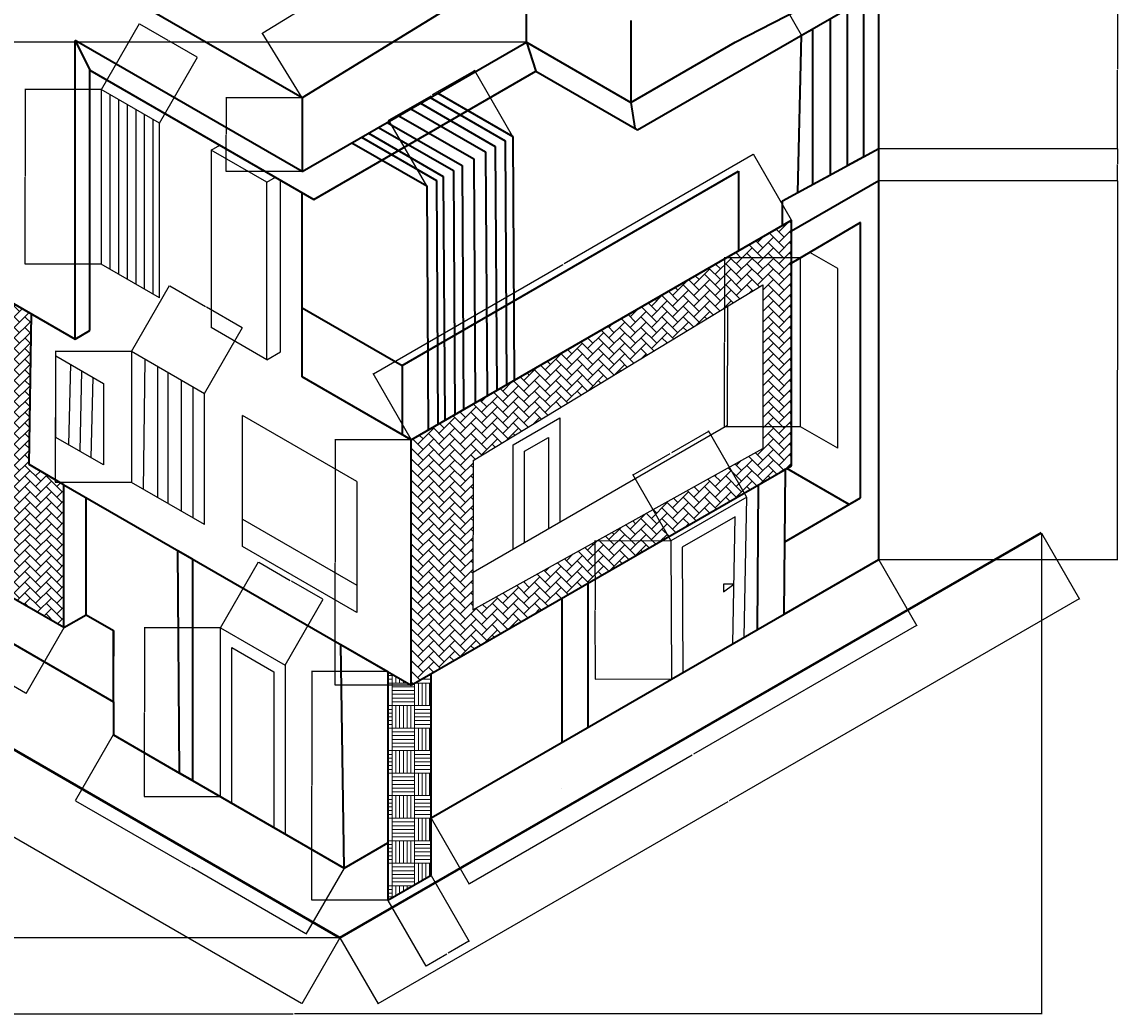
# Model space of a CAD drawing. Units: inches. Extents: x 61 to 939, y -128 to 676.
# Tile 2 of 3: x 355 to 939, y -128 to 400. Entities that reach past the tile are written whole.
import ezdxf

# ---------------------------------------------------------------- set-up
doc = ezdxf.new("R2010")
doc.units = ezdxf.units.IN
doc.header["$MEASUREMENT"] = 0
for name, color, linetype, lineweight in [('A-ANNO-DIMS', 2, 'Continuous', 18), ('A-DOOR', 3, 'Continuous', 25), ('A-ELEV', 7, 'Continuous', 35), ('A-GLAZ', 4, 'Continuous', 25), ('A-WALL-PATT', 8, 'Continuous', 18), ('C-TOPO', 7, 'Continuous', 50)]:
    doc.layers.add(name, color=color, linetype=linetype, lineweight=lineweight)
doc.styles.get("Standard").update_dxf_attribs({"font": 'arial.ttf'})
doc.dimstyles.get("Standard").update_dxf_attribs({"dimtxt": 0.18, "dimasz": 0.18, "dimexe": 0.18, "dimexo": 0.0625, "dimgap": 0.09, "dimtad": 0, "dimtih": 1, "dimtoh": 1, "dimdec": 4, "dimzin": 0, "dimdsep": 46, "dimtxsty": 'Standard', "dimcen": 0.09, "dimadec": 0, "dimazin": 0, "dimtfac": 1, "dimtdec": 4, "dimtofl": 0, "dimtmove": 0, "dimatfit": 3, "dimfxl": 1, "dimtolj": 1, "dimtzin": 0, "dimarcsym": 0})

# ---------------------------------------------------------------- blocks, each defined once
blk = doc.blocks.new('*D1')
at = {"layer": 'A-ANNO-DIMS', "color": 0, "lineweight": -2, "transparency": 16777216}
for p, q in [((273.62, 289.95), (273.62, 675.84)), ((273.8, 675.66), (542.03, 675.66)), ((811.05, 675.66), (542.82, 675.66)), ((811.23, 479.78), (811.23, 675.84))]:
    blk.add_line(p, q, dxfattribs=at)
at = {"layer": 'A-ANNO-DIMS', "color": 0, "transparency": 16777216}
for points in [[(273.8, 675.69), (273.8, 675.63), (273.62, 675.66)], [(811.05, 675.69), (811.05, 675.63), (811.23, 675.66)]]:
    blk.add_solid(points, dxfattribs=at)
at = {"layer": 'Defpoints', "color": 0, "transparency": 16777216}
for p in [(811.23, 675.66), (811.23, 479.72), (273.62, 289.89)]:
    blk.add_point(p, dxfattribs=at)
at = {"layer": 'A-ANNO-DIMS', "color": 0, "transparency": 16777216, "insert": (542.42, 675.66), "char_height": 0.18, "attachment_point": 5}
blk.add_mtext('\\A1;537.6', dxfattribs=at)
blk = doc.blocks.new('*D2')
at = {"layer": 'A-ANNO-DIMS', "color": 0, "lineweight": -2, "transparency": 16777216}
for p, q in [((541.93, 635.16), (60.74, 635.16)), ((60.92, 634.98), (60.92, 273.9)), ((60.92, -87.54), (60.92, 273.54)), ((524.15, -87.72), (60.74, -87.72))]:
    blk.add_line(p, q, dxfattribs=at)
at = {"layer": 'A-ANNO-DIMS', "color": 0, "transparency": 16777216}
for points in [[(60.89, 634.98), (60.95, 634.98), (60.92, 635.16)], [(60.89, -87.54), (60.95, -87.54), (60.92, -87.72)]]:
    blk.add_solid(points, dxfattribs=at)
at = {"layer": 'Defpoints', "color": 0, "transparency": 16777216}
for p in [(60.92, 635.16), (542, 635.16), (524.21, -87.72)]:
    blk.add_point(p, dxfattribs=at)
at = {"layer": 'A-ANNO-DIMS', "color": 0, "transparency": 16777216, "insert": (60.92, 273.72), "char_height": 0.18, "attachment_point": 5}
blk.add_mtext('\\A1;722.9', dxfattribs=at)
blk = doc.blocks.new('*D3')
at = {"layer": 'A-ANNO-DIMS', "color": 0, "lineweight": -2, "transparency": 16777216}
for p, q in [((101.42, 156.32), (101.42, -128.4)), ((897.89, 127.95), (897.89, -128.4)), ((101.6, -128.22), (499.26, -128.22)), ((897.71, -128.22), (500.04, -128.22))]:
    blk.add_line(p, q, dxfattribs=at)
at = {"layer": 'A-ANNO-DIMS', "color": 0, "transparency": 16777216}
for points in [[(101.6, -128.19), (101.6, -128.25), (101.42, -128.22)], [(897.71, -128.19), (897.71, -128.25), (897.89, -128.22)]]:
    blk.add_solid(points, dxfattribs=at)
at = {"layer": 'Defpoints', "color": 0, "transparency": 16777216}
for p in [(101.42, 156.38), (897.89, 128.02), (897.89, -128.22)]:
    blk.add_point(p, dxfattribs=at)
at = {"layer": 'A-ANNO-DIMS', "color": 0, "transparency": 16777216, "insert": (499.65, -128.22), "char_height": 0.18, "attachment_point": 5}
blk.add_mtext('\\A1;796.5', dxfattribs=at)
blk = doc.blocks.new('*D4')
at = {"layer": 'A-ANNO-DIMS', "color": 0, "lineweight": -2, "transparency": 16777216}
for p, q in [((811.29, 315.9), (938.57, 315.9)), ((938.39, 315.72), (938.39, 215.03)), ((938.39, 113.98), (938.39, 214.67)), ((811.29, 113.8), (938.57, 113.8))]:
    blk.add_line(p, q, dxfattribs=at)
at = {"layer": 'A-ANNO-DIMS', "color": 0, "transparency": 16777216}
for points in [[(938.36, 315.72), (938.42, 315.72), (938.39, 315.9)], [(938.36, 113.98), (938.42, 113.98), (938.39, 113.8)]]:
    blk.add_solid(points, dxfattribs=at)
at = {"layer": 'Defpoints', "color": 0, "transparency": 16777216}
for p in [(811.23, 315.9), (938.39, 315.9), (811.23, 113.8)]:
    blk.add_point(p, dxfattribs=at)
at = {"layer": 'A-ANNO-DIMS', "color": 0, "transparency": 16777216, "insert": (938.39, 214.85), "char_height": 0.18, "attachment_point": 5}
blk.add_mtext('\\A1;202.1', dxfattribs=at)
blk = doc.blocks.new('*D5')
at = {"layer": 'A-ANNO-DIMS', "color": 0, "lineweight": -2, "transparency": 16777216}
for p, q in [((811.29, 332.9), (938.57, 332.9)), ((938.39, 332.72), (938.39, 324.58)), ((938.39, 316.08), (938.39, 324.22)), ((811.29, 315.9), (938.57, 315.9))]:
    blk.add_line(p, q, dxfattribs=at)
at = {"layer": 'A-ANNO-DIMS', "color": 0, "transparency": 16777216}
for points in [[(938.36, 332.72), (938.42, 332.72), (938.39, 332.9)], [(938.36, 316.08), (938.42, 316.08), (938.39, 315.9)]]:
    blk.add_solid(points, dxfattribs=at)
at = {"layer": 'Defpoints', "color": 0, "transparency": 16777216}
for p in [(811.23, 332.9), (938.39, 332.9), (811.23, 315.9)]:
    blk.add_point(p, dxfattribs=at)
at = {"layer": 'A-ANNO-DIMS', "color": 0, "transparency": 16777216, "insert": (938.39, 324.4), "char_height": 0.18, "attachment_point": 5}
blk.add_mtext('\\A1;16.996', dxfattribs=at)
blk = doc.blocks.new('*D6')
at = {"layer": 'A-ANNO-DIMS', "color": 0, "lineweight": -2, "transparency": 16777216}
for p, q in [((811.29, 416.97), (938.57, 416.97)), ((938.39, 416.79), (938.39, 375.11)), ((938.39, 333.08), (938.39, 374.75)), ((811.29, 332.9), (938.57, 332.9))]:
    blk.add_line(p, q, dxfattribs=at)
at = {"layer": 'A-ANNO-DIMS', "color": 0, "transparency": 16777216}
for points in [[(938.36, 416.79), (938.42, 416.79), (938.39, 416.97)], [(938.36, 333.08), (938.42, 333.08), (938.39, 332.9)]]:
    blk.add_solid(points, dxfattribs=at)
at = {"layer": 'Defpoints', "color": 0, "transparency": 16777216}
for p in [(811.23, 416.97), (938.39, 416.97), (811.23, 332.9)]:
    blk.add_point(p, dxfattribs=at)
at = {"layer": 'A-ANNO-DIMS', "color": 0, "transparency": 16777216, "insert": (938.39, 374.93), "char_height": 0.18, "attachment_point": 5}
blk.add_mtext('\\A1;84.07', dxfattribs=at)
blk = doc.blocks.new('*D11')
at = {"layer": 'A-ANNO-DIMS', "color": 0, "lineweight": -2, "transparency": 16777216}
for p, q in [((549.64, 54.14), (509.02, 54.14)), ((509.2, 53.96), (509.2, -6.61)), ((509.2, -67.54), (509.2, -6.97)), ((549.64, -67.72), (509.02, -67.72))]:
    blk.add_line(p, q, dxfattribs=at)
at = {"layer": 'A-ANNO-DIMS', "color": 0, "transparency": 16777216}
for points in [[(509.17, 53.96), (509.23, 53.96), (509.2, 54.14)], [(509.17, -67.54), (509.23, -67.54), (509.2, -67.72)]]:
    blk.add_solid(points, dxfattribs=at)
at = {"layer": 'Defpoints', "color": 0, "transparency": 16777216}
for p in [(509.2, 54.14), (549.7, 54.14), (549.7, -67.72)]:
    blk.add_point(p, dxfattribs=at)
at = {"layer": 'A-ANNO-DIMS', "color": 0, "transparency": 16777216, "insert": (509.2, -6.79), "char_height": 0.18, "attachment_point": 5}
blk.add_mtext('\\A1;121.86', dxfattribs=at)
blk = doc.blocks.new('*D12')
at = {"layer": 'A-ANNO-DIMS', "color": 0, "lineweight": -2, "transparency": 16777216}
for p, q in [((562.18, 177.73), (521.56, 177.73)), ((521.74, 177.55), (521.74, 112.49)), ((521.74, 47.08), (521.74, 112.13)), ((562.18, 46.9), (521.56, 46.9))]:
    blk.add_line(p, q, dxfattribs=at)
at = {"layer": 'A-ANNO-DIMS', "color": 0, "transparency": 16777216}
for points in [[(521.71, 177.55), (521.77, 177.55), (521.74, 177.73)], [(521.71, 47.08), (521.77, 47.08), (521.74, 46.9)]]:
    blk.add_solid(points, dxfattribs=at)
at = {"layer": 'Defpoints', "color": 0, "transparency": 16777216}
for p in [(521.74, 177.73), (562.24, 177.73), (562.24, 46.9)]:
    blk.add_point(p, dxfattribs=at)
at = {"layer": 'A-ANNO-DIMS', "color": 0, "transparency": 16777216, "insert": (521.74, 112.31), "char_height": 0.18, "attachment_point": 5}
blk.add_mtext('\\A1;130.83', dxfattribs=at)
blk = doc.blocks.new('*D13')
at = {"layer": 'A-ANNO-DIMS', "color": 0, "lineweight": -2, "transparency": 16777216}
for p, q in [((504.12, 359.95), (463.5, 359.95)), ((463.68, 359.77), (463.68, 340.5)), ((463.68, 320.87), (463.68, 340.14)), ((504.12, 320.69), (463.5, 320.69))]:
    blk.add_line(p, q, dxfattribs=at)
at = {"layer": 'A-ANNO-DIMS', "color": 0, "transparency": 16777216}
for points in [[(463.65, 359.77), (463.71, 359.77), (463.68, 359.95)], [(463.65, 320.87), (463.71, 320.87), (463.68, 320.69)]]:
    blk.add_solid(points, dxfattribs=at)
at = {"layer": 'Defpoints', "color": 0, "transparency": 16777216}
for p in [(463.68, 359.95), (504.18, 359.95), (504.18, 320.69)]:
    blk.add_point(p, dxfattribs=at)
at = {"layer": 'A-ANNO-DIMS', "color": 0, "transparency": 16777216, "insert": (463.68, 340.32), "char_height": 0.18, "attachment_point": 5}
blk.add_mtext('\\A1;39.26', dxfattribs=at)
blk = doc.blocks.new('*D14')
at = {"layer": 'A-ANNO-DIMS', "color": 0, "lineweight": -2, "transparency": 16777216}
for p, q in [((460.53, 77.39), (419.91, 77.39)), ((420.09, 77.21), (420.09, 32.6)), ((420.09, -12.36), (420.09, 32.24)), ((460.53, -12.54), (419.91, -12.54))]:
    blk.add_line(p, q, dxfattribs=at)
at = {"layer": 'A-ANNO-DIMS', "color": 0, "transparency": 16777216}
for points in [[(420.06, 77.21), (420.12, 77.21), (420.09, 77.39)], [(420.06, -12.36), (420.12, -12.36), (420.09, -12.54)]]:
    blk.add_solid(points, dxfattribs=at)
at = {"layer": 'Defpoints', "color": 0, "transparency": 16777216}
for p in [(420.09, 77.39), (460.59, 77.39), (460.59, -12.54)]:
    blk.add_point(p, dxfattribs=at)
at = {"layer": 'A-ANNO-DIMS', "color": 0, "transparency": 16777216, "insert": (420.09, 32.42), "char_height": 0.18, "attachment_point": 5}
blk.add_mtext('\\A1;89.93', dxfattribs=at)
blk = doc.blocks.new('*D15')
at = {"layer": 'A-ANNO-DIMS', "color": 0, "lineweight": -2, "transparency": 16777216}
for p, q in [((460.62, 77.44), (480.93, 112.62)), ((481, 112.37), (497.74, 102.7)), ((515.12, 92.67), (498.37, 102.34)), ((495.06, 57.56), (515.37, 92.73))]:
    blk.add_line(p, q, dxfattribs=at)
at = {"layer": 'A-ANNO-DIMS', "color": 0, "transparency": 16777216}
for points in [[(481.01, 112.4), (480.98, 112.35), (480.84, 112.46)], [(515.14, 92.69), (515.11, 92.64), (515.28, 92.58)]]:
    blk.add_solid(points, dxfattribs=at)
at = {"layer": 'Defpoints', "color": 0, "transparency": 16777216}
for p in [(515.28, 92.58), (460.59, 77.39), (495.03, 57.5)]:
    blk.add_point(p, dxfattribs=at)
at = {"layer": 'A-ANNO-DIMS', "color": 0, "transparency": 16777216, "insert": (498.06, 102.52), "char_height": 0.18, "attachment_point": 5}
blk.add_mtext('\\A1;39.77', dxfattribs=at)
blk = doc.blocks.new('*D16')
at = {"layer": 'A-ANNO-DIMS', "color": 0, "lineweight": -2, "transparency": 16777216}
for p, q in [((700.49, 123.86), (659.87, 123.68)), ((660.05, 123.5), (660.21, 86.98)), ((660.37, 50.09), (660.21, 86.61)), ((700.81, 50.08), (660.19, 49.91))]:
    blk.add_line(p, q, dxfattribs=at)
at = {"layer": 'A-ANNO-DIMS', "color": 0, "transparency": 16777216}
for points in [[(660.08, 123.5), (660.02, 123.5), (660.05, 123.68)], [(660.4, 50.09), (660.34, 50.09), (660.37, 49.91)]]:
    blk.add_solid(points, dxfattribs=at)
at = {"layer": 'Defpoints', "color": 0, "transparency": 16777216}
for p in [(660.05, 123.68), (700.55, 123.86), (700.87, 50.08)]:
    blk.add_point(p, dxfattribs=at)
at = {"layer": 'A-ANNO-DIMS', "color": 0, "transparency": 16777216, "insert": (660.21, 86.8), "char_height": 0.18, "attachment_point": 5}
blk.add_mtext('\\A1;73.78', dxfattribs=at)
blk = doc.blocks.new('*D17')
at = {"layer": 'A-ANNO-DIMS', "color": 0, "lineweight": -2, "transparency": 16777216}
for p, q in [((720.52, 182.16), (700.81, 170.77)), ((740.9, 147.23), (720.59, 182.4)), ((680.46, 159.02), (700.18, 170.41)), ((700.52, 123.91), (680.21, 159.09))]:
    blk.add_line(p, q, dxfattribs=at)
at = {"layer": 'A-ANNO-DIMS', "color": 0, "transparency": 16777216}
for points in [[(720.51, 182.18), (720.54, 182.13), (720.68, 182.25)], [(680.44, 159.05), (680.47, 159), (680.3, 158.93)]]:
    blk.add_solid(points, dxfattribs=at)
at = {"layer": 'Defpoints', "color": 0, "transparency": 16777216}
for p in [(720.68, 182.25), (740.93, 147.17), (700.55, 123.86)]:
    blk.add_point(p, dxfattribs=at)
at = {"layer": 'A-ANNO-DIMS', "color": 0, "transparency": 16777216, "insert": (700.49, 170.59), "char_height": 0.18, "attachment_point": 5}
blk.add_mtext('\\A1;46.63', dxfattribs=at)
blk = doc.blocks.new('*D20')
at = {"layer": 'A-ANNO-DIMS', "color": 0, "lineweight": -2, "transparency": 16777216}
for p, q in [((397.03, 364.33), (356.42, 364.33)), ((356.6, 364.15), (356.6, 317.96)), ((356.6, 271.41), (356.6, 317.6)), ((397.03, 271.23), (356.42, 271.23))]:
    blk.add_line(p, q, dxfattribs=at)
at = {"layer": 'A-ANNO-DIMS', "color": 0, "transparency": 16777216}
for points in [[(356.57, 364.15), (356.63, 364.15), (356.6, 364.33)], [(356.57, 271.41), (356.63, 271.41), (356.6, 271.23)]]:
    blk.add_solid(points, dxfattribs=at)
at = {"layer": 'Defpoints', "color": 0, "transparency": 16777216}
for p in [(356.6, 364.33), (397.1, 364.33), (397.1, 271.23)]:
    blk.add_point(p, dxfattribs=at)
at = {"layer": 'A-ANNO-DIMS', "color": 0, "transparency": 16777216, "insert": (356.6, 317.78), "char_height": 0.18, "attachment_point": 5}
blk.add_mtext('\\A1;93.1', dxfattribs=at)
blk = doc.blocks.new('*D21')
at = {"layer": 'A-ANNO-DIMS', "color": 0, "lineweight": -2, "transparency": 16777216}
for p, q in [((397.13, 364.39), (417.44, 399.56)), ((417.5, 399.32), (432.53, 390.64)), ((448.19, 381.6), (433.16, 390.27)), ((428.13, 346.49), (448.44, 381.66))]:
    blk.add_line(p, q, dxfattribs=at)
at = {"layer": 'A-ANNO-DIMS', "color": 0, "transparency": 16777216}
for points in [[(417.52, 399.34), (417.49, 399.29), (417.35, 399.41)], [(448.21, 381.62), (448.18, 381.57), (448.35, 381.51)]]:
    blk.add_solid(points, dxfattribs=at)
at = {"layer": 'Defpoints', "color": 0, "transparency": 16777216}
for p in [(448.35, 381.51), (397.1, 364.33), (428.1, 346.43)]:
    blk.add_point(p, dxfattribs=at)
at = {"layer": 'A-ANNO-DIMS', "color": 0, "transparency": 16777216, "insert": (432.85, 390.46), "char_height": 0.18, "attachment_point": 5}
blk.add_mtext('\\A1;35.8', dxfattribs=at)
blk = doc.blocks.new('*D22')
at = {"layer": 'A-ANNO-DIMS', "color": 0, "lineweight": -2, "transparency": 16777216}
for p, q in [((413.11, 224.66), (372.49, 224.66)), ((372.67, 224.48), (372.67, 189.96)), ((372.67, 155.07), (372.67, 189.59)), ((413.11, 154.89), (372.49, 154.89))]:
    blk.add_line(p, q, dxfattribs=at)
at = {"layer": 'A-ANNO-DIMS', "color": 0, "transparency": 16777216}
for points in [[(372.64, 224.48), (372.7, 224.48), (372.67, 224.66)], [(372.64, 155.07), (372.7, 155.07), (372.67, 154.89)]]:
    blk.add_solid(points, dxfattribs=at)
at = {"layer": 'Defpoints', "color": 0, "transparency": 16777216}
for p in [(372.67, 224.66), (413.17, 224.66), (413.17, 154.89)]:
    blk.add_point(p, dxfattribs=at)
at = {"layer": 'A-ANNO-DIMS', "color": 0, "transparency": 16777216, "insert": (372.67, 189.78), "char_height": 0.18, "attachment_point": 5}
blk.add_mtext('\\A1;69.77', dxfattribs=at)
blk = doc.blocks.new('*D23')
at = {"layer": 'A-ANNO-DIMS', "color": 0, "lineweight": -2, "transparency": 16777216}
for p, q in [((413.2, 224.71), (433.51, 259.89)), ((433.58, 259.64), (452.54, 248.7)), ((472.12, 237.39), (453.17, 248.34)), ((452.06, 202.28), (472.37, 237.46))]:
    blk.add_line(p, q, dxfattribs=at)
at = {"layer": 'A-ANNO-DIMS', "color": 0, "transparency": 16777216}
for points in [[(433.59, 259.67), (433.56, 259.62), (433.42, 259.73)], [(472.14, 237.42), (472.11, 237.36), (472.28, 237.3)]]:
    blk.add_solid(points, dxfattribs=at)
at = {"layer": 'Defpoints', "color": 0, "transparency": 16777216}
for p in [(472.28, 237.3), (413.17, 224.66), (452.03, 202.23)]:
    blk.add_point(p, dxfattribs=at)
at = {"layer": 'A-ANNO-DIMS', "color": 0, "transparency": 16777216, "insert": (452.85, 248.52), "char_height": 0.18, "attachment_point": 5}
blk.add_mtext('\\A1;44.87', dxfattribs=at)
blk = doc.blocks.new('*D24')
at = {"layer": 'A-ANNO-DIMS', "color": 0, "lineweight": -2, "transparency": 16777216}
for p, q in [((769.5, 274.61), (728.89, 274.61)), ((729.07, 274.43), (729.07, 229.81)), ((729.07, 184.84), (729.07, 229.45)), ((769.5, 184.66), (728.89, 184.66))]:
    blk.add_line(p, q, dxfattribs=at)
at = {"layer": 'A-ANNO-DIMS', "color": 0, "transparency": 16777216}
for points in [[(729.04, 274.43), (729.1, 274.43), (729.07, 274.61)], [(729.04, 184.84), (729.1, 184.84), (729.07, 184.66)]]:
    blk.add_solid(points, dxfattribs=at)
at = {"layer": 'Defpoints', "color": 0, "transparency": 16777216}
for p in [(729.07, 274.61), (769.57, 274.61), (769.57, 184.66)]:
    blk.add_point(p, dxfattribs=at)
at = {"layer": 'A-ANNO-DIMS', "color": 0, "transparency": 16777216, "insert": (729.07, 229.63), "char_height": 0.18, "attachment_point": 5}
blk.add_mtext('\\A1;89.95', dxfattribs=at)
blk = doc.blocks.new('*D25')
at = {"layer": 'A-ANNO-DIMS', "color": 0, "lineweight": -2, "transparency": 16777216}
for p, q in [((744.42, 329.67), (643.6, 271.46)), ((764.8, 294.74), (744.49, 329.92)), ((542.15, 212.89), (642.97, 271.1)), ((562.21, 177.78), (541.9, 212.96))]:
    blk.add_line(p, q, dxfattribs=at)
at = {"layer": 'A-ANNO-DIMS', "color": 0, "transparency": 16777216}
for points in [[(744.41, 329.7), (744.44, 329.65), (744.58, 329.76)], [(542.13, 212.92), (542.16, 212.86), (541.99, 212.8)]]:
    blk.add_solid(points, dxfattribs=at)
at = {"layer": 'Defpoints', "color": 0, "transparency": 16777216}
for p in [(744.58, 329.76), (764.83, 294.69), (562.24, 177.73)]:
    blk.add_point(p, dxfattribs=at)
at = {"layer": 'A-ANNO-DIMS', "color": 0, "transparency": 16777216, "insert": (643.29, 271.28), "char_height": 0.18, "attachment_point": 5}
blk.add_mtext('\\A1;233.9', dxfattribs=at)
blk = doc.blocks.new('*D26')
at = {"layer": 'A-ANNO-DIMS', "color": 0, "lineweight": -2, "transparency": 16777216}
for p, q in [((101.38, 156.32), (81.08, 121.15)), ((81.32, 121.21), (292.25, -0.57)), ((503.81, -122.71), (292.88, -0.93)), ((524.18, -87.78), (503.87, -122.95))]:
    blk.add_line(p, q, dxfattribs=at)
at = {"layer": 'A-ANNO-DIMS', "color": 0, "transparency": 16777216}
for points in [[(81.34, 121.24), (81.31, 121.19), (81.17, 121.3)], [(503.82, -122.68), (503.79, -122.73), (503.96, -122.8)]]:
    blk.add_solid(points, dxfattribs=at)
at = {"layer": 'Defpoints', "color": 0, "transparency": 16777216}
for p in [(101.42, 156.38), (81.17, 121.3), (524.21, -87.72)]:
    blk.add_point(p, dxfattribs=at)
at = {"layer": 'A-ANNO-DIMS', "color": 0, "transparency": 16777216, "insert": (292.56, -0.75), "char_height": 0.18, "attachment_point": 5}
blk.add_mtext('\\A1;488.20', dxfattribs=at)
blk = doc.blocks.new('*D27')
at = {"layer": 'A-ANNO-DIMS', "color": 0, "lineweight": -2, "transparency": 16777216}
for p, q in [((897.92, 127.96), (918.23, 92.79)), ((917.98, 92.85), (731.61, -14.75)), ((544.62, -122.71), (730.98, -15.11)), ((524.24, -87.78), (544.55, -122.95))]:
    blk.add_line(p, q, dxfattribs=at)
at = {"layer": 'A-ANNO-DIMS', "color": 0, "transparency": 16777216}
for points in [[(917.97, 92.88), (918, 92.83), (918.14, 92.94)], [(544.6, -122.68), (544.63, -122.73), (544.46, -122.8)]]:
    blk.add_solid(points, dxfattribs=at)
at = {"layer": 'Defpoints', "color": 0, "transparency": 16777216}
for p in [(897.89, 128.02), (524.21, -87.72), (544.46, -122.8)]:
    blk.add_point(p, dxfattribs=at)
at = {"layer": 'A-ANNO-DIMS', "color": 0, "transparency": 16777216, "insert": (731.3, -14.93), "char_height": 0.18, "attachment_point": 5}
blk.add_mtext('\\A1;431.48', dxfattribs=at)
blk = doc.blocks.new('*D30')
at = {"layer": 'A-ANNO-DIMS', "color": 0, "lineweight": -2, "transparency": 16777216}
for p, q in [((602.19, 467.71), (542.96, 431.31)), ((623.52, 433.36), (602.25, 467.96)), ((483.13, 394.55), (542.37, 430.95)), ((504.15, 360), (482.88, 394.61))]:
    blk.add_line(p, q, dxfattribs=at)
at = {"layer": 'A-ANNO-DIMS', "color": 0, "transparency": 16777216}
for points in [[(602.17, 467.74), (602.21, 467.69), (602.34, 467.81)], [(483.12, 394.58), (483.15, 394.52), (482.98, 394.46)]]:
    blk.add_solid(points, dxfattribs=at)
at = {"layer": 'Defpoints', "color": 0, "transparency": 16777216}
for p in [(602.34, 467.81), (623.55, 433.3), (504.18, 359.95)]:
    blk.add_point(p, dxfattribs=at)
at = {"layer": 'A-ANNO-DIMS', "color": 0, "transparency": 16777216, "insert": (542.66, 431.13), "char_height": 0.18, "attachment_point": 5}
blk.add_mtext('\\A1;140.10', dxfattribs=at)
blk = doc.blocks.new('*D32')
at = {"layer": 'A-ANNO-DIMS', "color": 0, "lineweight": -2, "transparency": 16777216}
for p, q in [((623.49, 433.3), (60.74, 433.3)), ((60.92, 433.12), (60.92, 411.64)), ((60.92, 389.79), (60.92, 411.27)), ((623.49, 389.61), (60.74, 389.61))]:
    blk.add_line(p, q, dxfattribs=at)
at = {"layer": 'A-ANNO-DIMS', "color": 0, "transparency": 16777216}
for points in [[(60.89, 433.12), (60.95, 433.12), (60.92, 433.3)], [(60.89, 389.79), (60.95, 389.79), (60.92, 389.61)]]:
    blk.add_solid(points, dxfattribs=at)
at = {"layer": 'Defpoints', "color": 0, "transparency": 16777216}
for p in [(623.55, 433.3), (60.92, 389.61), (623.55, 389.61)]:
    blk.add_point(p, dxfattribs=at)
at = {"layer": 'A-ANNO-DIMS', "color": 0, "transparency": 16777216, "insert": (60.92, 411.46), "char_height": 0.18, "attachment_point": 5}
blk.add_mtext('\\A1;43.695', dxfattribs=at)
blk = doc.blocks.new('*D33')
at = {"layer": 'A-ANNO-DIMS', "color": 0, "lineweight": -2, "transparency": 16777216}
for p, q in [((403.49, 20.35), (383.18, -14.82)), ((383.43, -14.76), (444.44, -49.99)), ((506.09, -85.58), (445.07, -50.35)), ((526.46, -50.65), (506.15, -85.82))]:
    blk.add_line(p, q, dxfattribs=at)
at = {"layer": 'A-ANNO-DIMS', "color": 0, "transparency": 16777216}
for points in [[(383.44, -14.73), (383.41, -14.78), (383.27, -14.67)], [(506.1, -85.55), (506.07, -85.6), (506.24, -85.67)]]:
    blk.add_solid(points, dxfattribs=at)
at = {"layer": 'Defpoints', "color": 0, "transparency": 16777216}
for p in [(403.52, 20.41), (383.27, -14.67), (526.49, -50.59)]:
    blk.add_point(p, dxfattribs=at)
at = {"layer": 'A-ANNO-DIMS', "color": 0, "transparency": 16777216, "insert": (444.76, -50.17), "char_height": 0.18, "attachment_point": 5}
blk.add_mtext('\\A1;142.00', dxfattribs=at)
blk = doc.blocks.new('*D34')
at = {"layer": 'A-ANNO-DIMS', "color": 0, "lineweight": -2, "transparency": 16777216}
for p, q in [((811.26, 113.75), (831.57, 78.57)), ((831.32, 78.64), (712.57, 10.07)), ((593.18, -58.86), (711.94, 9.71)), ((572.8, -23.93), (593.11, -59.1))]:
    blk.add_line(p, q, dxfattribs=at)
at = {"layer": 'A-ANNO-DIMS', "color": 0, "transparency": 16777216}
for points in [[(831.31, 78.66), (831.34, 78.61), (831.48, 78.73)], [(593.16, -58.83), (593.19, -58.88), (593.02, -58.95)]]:
    blk.add_solid(points, dxfattribs=at)
at = {"layer": 'Defpoints', "color": 0, "transparency": 16777216}
for p in [(811.23, 113.8), (572.77, -23.87), (593.02, -58.95)]:
    blk.add_point(p, dxfattribs=at)
at = {"layer": 'A-ANNO-DIMS', "color": 0, "transparency": 16777216, "insert": (712.25, 9.89), "char_height": 0.18, "attachment_point": 5}
blk.add_mtext('\\A1;275.35', dxfattribs=at)
blk = doc.blocks.new('*D35')
at = {"layer": 'A-ANNO-DIMS', "color": 0, "lineweight": -2, "transparency": 16777216}
for p, q in [((595.86, 374.38), (573.44, 361.44)), ((616.24, 339.45), (595.93, 374.63)), ((550.4, 348.13), (572.81, 361.07)), ((570.46, 313.02), (550.15, 348.2))]:
    blk.add_line(p, q, dxfattribs=at)
at = {"layer": 'A-ANNO-DIMS', "color": 0, "transparency": 16777216}
for points in [[(595.85, 374.41), (595.88, 374.35), (596.02, 374.47)], [(550.38, 348.16), (550.41, 348.1), (550.24, 348.04)]]:
    blk.add_solid(points, dxfattribs=at)
at = {"layer": 'Defpoints', "color": 0, "transparency": 16777216}
for p in [(596.02, 374.47), (616.27, 339.4), (570.49, 312.97)]:
    blk.add_point(p, dxfattribs=at)
at = {"layer": 'A-ANNO-DIMS', "color": 0, "transparency": 16777216, "insert": (573.13, 361.25), "char_height": 0.18, "attachment_point": 5}
blk.add_mtext('\\A1;52.86', dxfattribs=at)
blk = doc.blocks.new('*D36')
at = {"layer": 'A-ANNO-DIMS', "color": 0, "lineweight": -2, "transparency": 16777216}
for p, q in [((572.8, -54.46), (593.11, -89.63)), ((549.73, -67.78), (570.04, -102.95)), ((592.87, -89.57), (581.8, -95.96)), ((570.11, -102.71), (581.17, -96.32))]:
    blk.add_line(p, q, dxfattribs=at)
at = {"layer": 'A-ANNO-DIMS', "color": 0, "transparency": 16777216}
for points in [[(592.85, -89.54), (592.88, -89.59), (593.02, -89.48)], [(570.09, -102.68), (570.12, -102.73), (569.95, -102.8)]]:
    blk.add_solid(points, dxfattribs=at)
at = {"layer": 'Defpoints', "color": 0, "transparency": 16777216}
for p in [(572.77, -54.4), (549.7, -67.72), (569.95, -102.8)]:
    blk.add_point(p, dxfattribs=at)
at = {"layer": 'A-ANNO-DIMS', "color": 0, "transparency": 16777216, "insert": (581.49, -96.14), "char_height": 0.18, "attachment_point": 5}
blk.add_mtext('\\A1;26.643', dxfattribs=at)
blk = doc.blocks.new('*D37')
at = {"layer": 'A-ANNO-DIMS', "color": 0, "lineweight": -2, "transparency": 16777216}
for p, q in [((325.55, 107.3), (305.24, 72.12)), ((377.15, 77.51), (356.84, 42.33)), ((305.48, 72.19), (330.81, 57.56)), ((356.77, 42.58), (331.44, 57.2))]:
    blk.add_line(p, q, dxfattribs=at)
at = {"layer": 'A-ANNO-DIMS', "color": 0, "transparency": 16777216}
for points in [[(305.5, 72.21), (305.47, 72.16), (305.33, 72.28)], [(356.79, 42.6), (356.76, 42.55), (356.93, 42.49)]]:
    blk.add_solid(points, dxfattribs=at)
at = {"layer": 'Defpoints', "color": 0, "transparency": 16777216}
for p in [(325.58, 107.35), (377.18, 77.56), (305.33, 72.28)]:
    blk.add_point(p, dxfattribs=at)
at = {"layer": 'A-ANNO-DIMS', "color": 0, "transparency": 16777216, "insert": (331.13, 57.38), "char_height": 0.18, "attachment_point": 5}
blk.add_mtext('\\A1;59.58', dxfattribs=at)
blk = doc.blocks.new('*D38')
at = {"layer": 'A-ANNO-DIMS', "color": 0, "lineweight": -2, "transparency": 16777216}
for p, q in [((782.94, 447.4), (766.82, 438.09)), ((803.31, 412.47), (783, 447.65)), ((750.07, 428.42), (766.19, 437.73)), ((770.13, 393.31), (749.82, 428.49))]:
    blk.add_line(p, q, dxfattribs=at)
at = {"layer": 'A-ANNO-DIMS', "color": 0, "transparency": 16777216}
for points in [[(782.92, 447.43), (782.95, 447.37), (783.09, 447.49)], [(750.06, 428.45), (750.09, 428.4), (749.91, 428.33)]]:
    blk.add_solid(points, dxfattribs=at)
at = {"layer": 'Defpoints', "color": 0, "transparency": 16777216}
for p in [(783.09, 447.49), (803.34, 412.42), (770.16, 393.26)]:
    blk.add_point(p, dxfattribs=at)
at = {"layer": 'A-ANNO-DIMS', "color": 0, "transparency": 16777216, "insert": (766.5, 437.91), "char_height": 0.18, "attachment_point": 5}
blk.add_mtext('\\A1;38.31', dxfattribs=at)

msp = doc.modelspace()

# ---------------------------------------------------------------- hatches: boundary and pattern name
at = {"layer": 'A-WALL-PATT'}
h = msp.add_hatch(dxfattribs=at)
h.set_pattern_fill('AR-HBONE', color=256)
h.paths.add_polyline_path([(764.8272, 163.8587), (764.8272, 294.6874), (562.2436, 177.7257), (562.2436, 46.897)])
h.paths.add_polyline_path([(595.2101, 166.7105), (749.5189, 260.1923), (749.5189, 172.9507), (595.1042, 87.0956)], flags=16)
h.paths.add_polyline_path([(377.1796, 153.7437), (358.6559, 164.4384), (359.9295, 244.7895), (325.5788, 264.6219), (325.5788, 215.6029), (325.5788, 131.6029), (325.5788, 107.3524), (377.1796, 77.5607)])
h = msp.add_hatch(dxfattribs=at)
h.set_pattern_fill('AR-PARQ1', color=256)
h.paths.add_polyline_path([(572.7731, 46.897), (572.7731, 52.9761), (562.2436, 46.897), (549.6993, 54.1394), (549.6993, -67.7244), (572.7731, -54.4028)])

# ---------------------------------------------------------------- linework, layer by layer
at = {"layer": 'A-DOOR'}
for p, q in [((728.608, 100.7561), (728.608, 96.7136)), ((728.608, 96.7136), (734.0855, 100.7561)), ((734.0855, 100.7561), (728.608, 100.7561))]:
    msp.add_line(p, q, dxfattribs=at)
for points in [[(616.5781, 119.4483), (616.5781, 175.0017), (641.347, 189.3021), (641.347, 133.7487)], [(622.5781, 122.9124), (622.5781, 171.5376), (635.347, 178.9097), (635.347, 130.2846)], [(739.5713, 72.4275), (740.9306, 147.1737), (700.5503, 123.8602), (700.8719, 50.0844)], [(733.5067, 68.926), (734.7386, 136.6706), (706.5655, 120.4048), (706.8569, 53.5398)], [(460.5892, -12.5431), (460.5892, 77.388), (495.0283, 57.5046), (495.0283, -32.4265)], [(466.5892, -16.0072), (466.5892, 66.9957), (489.0283, 54.0405), (489.0283, -28.9624)]]:
    msp.add_lwpolyline(points, dxfattribs=at)
at = {"layer": 'A-ELEV'}
for p, q in [((504.1826, 359.9507), (325.5788, 463.0676)), ((623.5481, 433.303), (504.1826, 359.9507)), ((623.5481, 389.6079), (623.5481, 433.303)), ((734.7429, 389.6058), (811.2295, 429.2088)), ((811.2295, 113.7993), (811.2295, 429.2088)), ((752.0802, 382.8189), (811.2295, 416.9688)), ((803.3445, 328.6095), (803.3445, 412.4164)), ((794.4408, 407.2759), (794.4408, 323.7678)), ((679.1474, 401.2027), (679.1474, 357.5076)), ((785.5849, 318.9521), (785.5849, 402.1629)), ((768.1877, 309.4917), (770.1647, 393.2601)), ((770.1647, 393.2601), (775.9309, 396.5892)), ((775.9309, 396.5892), (775.9309, 313.7023)), ((383.2216, 231.3418), (383.2216, 390.529)), ((504.1826, 320.6921), (383.2216, 390.529)), ((383.2216, 390.529), (391.0622, 374.6784)), ((504.1826, 320.6921), (623.5481, 389.6079)), ((623.5481, 389.6079), (679.1474, 357.5076)), ((623.5481, 389.6079), (628.6401, 374.1046)), ((679.1474, 357.5076), (734.7429, 389.6058)), ((682.8133, 342.8277), (752.0802, 382.8189)), ((391.0622, 235.8686), (391.0622, 374.6784)), ((391.0622, 374.6784), (510.348, 305.8086)), ((510.348, 305.8086), (628.6401, 374.1046)), ((628.6401, 374.1046), (682.8133, 342.8277)), ((576.4219, 362.3995), (616.2663, 339.3954)), ((504.1826, 359.9507), (504.1826, 320.6921)), ((567.0994, 357.0172), (606.9438, 334.0131)), ((572.3294, 360.0367), (612.1737, 337.0326)), ((679.1474, 357.5076), (681.3042, 343.699)), ((555.6638, 350.4148), (595.5081, 327.4107)), ((555.6638, 350.4148), (595.5081, 327.4107)), ((562.0123, 354.0801), (601.8566, 331.076)), ((549.4352, 346.8187), (589.2795, 323.8146)), ((535.7946, 338.9433), (575.6389, 315.9392)), ((539.4562, 341.0573), (579.3005, 318.0532)), ((544.8393, 344.1653), (584.6836, 321.1611)), ((616.2663, 339.3954), (617.096, 209.3948)), ((530.6452, 335.9703), (570.4895, 312.9662)), ((606.9438, 334.0131), (607.7735, 204.0125)), ((612.1737, 337.0326), (613.0035, 207.032)), ((759.9403, 305.0069), (811.2295, 332.8972)), ((595.5081, 327.4107), (596.3379, 197.4101)), ((595.5081, 327.4107), (596.3379, 197.4101)), ((601.8566, 331.076), (602.6864, 201.0754)), ((794.4408, 323.7678), (803.3445, 328.6095)), ((589.2795, 323.8146), (590.1093, 193.814)), ((557.3797, 217.3286), (736.574, 320.7865)), ((575.6389, 315.9392), (576.4687, 185.9386)), ((579.3005, 318.0532), (580.1303, 188.0526)), ((584.6836, 321.1611), (585.5134, 191.1605)), ((736.574, 320.7865), (736.574, 278.3754)), ((764.8272, 289.1106), (811.2295, 315.9009)), ((775.9309, 313.7023), (785.5849, 318.9521)), ((570.4895, 312.9662), (571.3193, 182.9656)), ((504.1826, 211.2473), (504.1826, 309.3683)), ((759.9403, 291.866), (759.9403, 305.0069)), ((562.2436, 177.7257), (764.8272, 294.6874)), ((764.8272, 163.8587), (764.8272, 294.6874)), ((801.6305, 293.4263), (764.8272, 271.8242)), ((801.6305, 146.6822), (801.6305, 293.4263)), ((325.5788, 264.6219), (383.2216, 231.3418)), ((504.1826, 248.042), (557.3797, 217.3286)), ((358.6559, 164.4384), (359.9295, 244.7895)), ((383.2216, 231.3418), (391.0622, 235.8686)), ((557.3797, 217.3286), (557.3797, 180.5339)), ((562.2436, 177.7257), (504.1826, 211.2473)), ((562.2436, 46.897), (562.2436, 177.7257)), ((377.1796, 153.7437), (358.6559, 164.4384)), ((562.2436, 46.897), (764.8272, 163.8587)), ((761.6316, 162.0137), (758.6837, 160.3117)), ((760.7976, 84.6824), (761.6316, 162.0137)), ((795.4916, 143.1379), (762.2147, 162.3503)), ((377.1796, 77.5607), (377.1796, 153.7437)), ((377.1796, 153.7437), (562.2436, 46.897)), ((747.0486, 153.5942), (746.5734, 76.4701)), ((389.0714, 84.4264), (389.0714, 146.878)), ((761.2146, 123.3481), (801.6305, 146.6822)), ((438.7184, 0.084), (437.8165, 118.735)), ((437.8165, 118.735), (445.7748, 114.1403)), ((445.7748, 114.1403), (445.7748, -3.99)), ((760.7976, 84.6824), (811.2295, 113.7993)), ((377.1796, 77.5607), (325.5788, 107.3524)), ((656.2888, 101.194), (656.2888, 24.3443)), ((299.5981, 98.102), (403.5211, 38.102)), ((642.3895, 93.1692), (642.3895, 35.5373)), ((377.1796, 77.5607), (389.0714, 84.4264)), ((389.0714, 84.4264), (403.5211, 76.0839)), ((572.7731, -23.8735), (760.7976, 84.6824)), ((403.5211, 38.102), (403.5211, 76.0839)), ((403.5211, 76.0839), (403.5211, 62.3524)), ((526.4936, -50.593), (524.7335, 68.5535)), ((524.7335, 68.5535), (549.6993, 54.1394)), ((549.6993, 54.1394), (549.6993, -67.7244)), ((572.7731, 46.897), (572.7731, 52.9761)), ((572.7731, -54.4028), (572.7731, 46.897)), ((403.5211, 38.102), (403.5211, 20.4052)), ((642.3895, 35.5373), (642.3895, 16.3195)), ((403.5211, 20.4052), (438.7184, 0.084)), ((445.7748, -3.99), (438.7184, 0.084)), ((438.7184, 0.084), (445.7748, -3.99)), ((445.7748, -3.99), (526.4936, -50.593)), ((642.3895, -8.2416), (642.3895, -8.2416)), ((526.4936, -50.593), (549.6993, -37.1952)), ((549.6993, -67.7244), (572.7731, -54.4028))]:
    msp.add_line(p, q, dxfattribs=at)
at = {"layer": 'A-GLAZ'}
for p, q in [((428.0999, 346.432), (397.0972, 364.3314)), ((397.0972, 364.3314), (397.0972, 271.2304)), ((401.6801, 361.6855), (401.6801, 268.5845)), ((406.2631, 359.0395), (406.2631, 265.9385)), ((410.846, 356.3936), (410.846, 263.2925)), ((415.4289, 353.7476), (415.4289, 260.6466)), ((420.0119, 351.1016), (420.0119, 258.0006)), ((424.5948, 348.4557), (424.5948, 255.3547)), ((428.0999, 253.331), (428.0999, 346.432)), ((455.5909, 332.1091), (460.1926, 334.7659)), ((485.2637, 314.9775), (455.5909, 332.1091)), ((455.5909, 332.1091), (455.5909, 237.4591)), ((485.2637, 314.9775), (489.8654, 317.6343)), ((492.498, 224.5042), (492.498, 316.1144)), ((485.2637, 220.3275), (485.2637, 314.9775)), ((769.5663, 184.659), (769.5663, 274.6059)), ((789.4196, 269.0123), (774.6069, 277.5645)), ((428.0999, 253.331), (397.0972, 271.2304)), ((789.4196, 173.1966), (789.4196, 269.0123)), ((595.2101, 166.7105), (749.5189, 260.1923)), ((749.5189, 260.1923), (749.5189, 172.9507)), ((730.7724, 185.3784), (730.8619, 248.8897)), ((485.2637, 220.3275), (455.5909, 237.4591)), ((372.8777, 178.9449), (372.8777, 222.4144)), ((372.8777, 222.4144), (398.2983, 207.7378)), ((452.029, 202.2263), (413.1729, 224.6598)), ((413.1729, 224.6598), (413.1729, 154.8909)), ((485.2637, 220.3275), (492.498, 224.5042)), ((380.7177, 217.888), (379.7167, 174.9964)), ((420.3149, 220.5364), (419.3801, 151.3072)), ((426.9885, 216.6834), (426.9885, 146.9145)), ((386.5891, 214.4981), (385.588, 171.6066)), ((392.6094, 211.0223), (391.6084, 168.1308)), ((432.601, 213.443), (432.601, 143.6742)), ((398.2983, 207.7378), (398.2983, 164.2683)), ((439.6598, 209.3676), (439.6598, 139.5988)), ((445.8932, 205.7687), (445.8932, 135.9999)), ((452.029, 132.4574), (452.029, 202.2263)), ((472.2598, 120.7771), (472.2598, 190.546)), ((533.2131, 155.3546), (472.2598, 190.546)), ((595.1308, 107.0657), (730.7724, 185.3784)), ((789.4196, 173.1966), (769.5663, 184.659)), ((398.2983, 164.2683), (372.8777, 178.9449)), ((595.1042, 87.0956), (749.5189, 172.9507)), ((595.2101, 166.7105), (595.1042, 87.0956)), ((452.029, 132.4574), (413.1729, 154.8909)), ((533.2131, 155.3546), (533.2131, 85.5857)), ((472.2598, 135.3176), (533.2131, 100.1262)), ((533.2131, 85.5857), (472.2598, 120.7771))]:
    msp.add_line(p, q, dxfattribs=at)
at = {"layer": 'C-TOPO'}
for q in [(101.4156, 156.3775), (897.8863, 128.0168)]:
    msp.add_line((524.212, -87.7241), q, dxfattribs=at)

# ---------------------------------------------------------------- dimensions: what is measured, and where the dimension line sits
at = {"layer": 'A-ANNO-DIMS'}
for base, p1, p2, picture, middle in [((811.2295, 675.6599), (273.6173, 289.886), (811.2295, 479.7174), '*D1', (542.4234, 675.6599)), ((897.8863, -128.2241), (101.4156, 156.3775), (897.8863, 128.0168), '*D3', (499.6509, -128.2241))]:
    dim = msp.add_linear_dim(base=base, p1=p1, p2=p2, dimstyle='Standard', override={"dimdec": 1, "dimlfac": 1, "dimrnd": 0, "dimzin": 0, "dimdsep": 46, "dimlunit": 2}, dxfattribs=at)
    dim.commit()
    dim.dimension.update_dxf_attribs({"geometry": picture, "text_midpoint": middle})
for base, p1, p2, angle, override, picture, middle in [((60.9156, 635.1599), (524.212, -87.7241), (541.9952, 635.1599), 90, {"dimdec": 1, "dimlfac": 1, "dimrnd": 0, "dimzin": 0, "dimdsep": 46, "dimlunit": 2}, '*D2', (60.9156, 273.7179)), ((602.3439, 467.8085), (504.1826, 359.9507), (623.5481, 433.303), 31.5714469, {"dimdec": 2, "dimlfac": 1, "dimrnd": 0, "dimzin": 0, "dimdsep": 46, "dimlunit": 2}, '*D30', (542.6611, 431.1324)), ((783.0945, 447.4905), (770.1647, 393.2601), (803.3445, 412.4164), 30, {"dimdec": 2, "dimlfac": 1, "dimrnd": 0, "dimzin": 0, "dimdsep": 46, "dimlunit": 2}, '*D38', (766.5046, 437.9123)), ((60.9156, 389.6079), (623.5481, 433.303), (623.5481, 389.6079), 90, {"dimdec": 3, "dimlfac": 1, "dimrnd": 0, "dimzin": 0, "dimdsep": 46, "dimlunit": 2}, '*D32', (60.9156, 411.4554)), ((938.3863, 416.9688), (811.2295, 332.8972), (811.2295, 416.9688), 90, {"dimdec": 2, "dimlfac": 1, "dimrnd": 0, "dimzin": 0, "dimdsep": 46, "dimlunit": 2}, '*D6', (938.3863, 374.933)), ((448.3499, 381.506), (397.0972, 364.3314), (428.0999, 346.432), 330, {"dimdec": 1, "dimlfac": 1, "dimrnd": 0, "dimzin": 0, "dimdsep": 46, "dimlunit": 2}, '*D21', (432.8486, 390.4558)), ((596.0163, 374.4694), (570.4895, 312.9662), (616.2663, 339.3954), 30, {"dimdec": 2, "dimlfac": 1, "dimrnd": 0, "dimzin": 0, "dimdsep": 46, "dimlunit": 2}, '*D35', (573.1279, 361.2548)), ((356.5972, 364.3314), (397.0972, 271.2304), (397.0972, 364.3314), 90, {"dimdec": 1, "dimlfac": 1, "dimrnd": 0, "dimzin": 0, "dimdsep": 46, "dimlunit": 2}, '*D20', (356.5972, 317.7809)), ((463.6826, 359.9507), (504.1826, 320.6921), (504.1826, 359.9507), 90, {"dimdec": 2, "dimlfac": 1, "dimrnd": 0, "dimzin": 0, "dimdsep": 46, "dimlunit": 2}, '*D13', (463.6826, 340.3214)), ((938.3863, 332.8972), (811.2295, 315.9009), (811.2295, 332.8972), 90, {"dimdec": 3, "dimlfac": 1, "dimrnd": 0, "dimzin": 0, "dimdsep": 46, "dimlunit": 2}, '*D5', (938.3863, 324.3991)), ((744.5772, 329.7615), (562.2436, 177.7257), (764.8272, 294.6874), 30, {"dimdec": 1, "dimlfac": 1, "dimrnd": 0, "dimzin": 0, "dimdsep": 46, "dimlunit": 2}, '*D25', (643.2854, 271.2806)), ((938.3863, 315.9009), (811.2295, 113.7993), (811.2295, 315.9009), 90, {"dimdec": 1, "dimlfac": 1, "dimrnd": 0, "dimzin": 0, "dimdsep": 46, "dimlunit": 2}, '*D4', (938.3863, 214.8501)), ((729.0663, 274.6059), (769.5663, 184.659), (769.5663, 274.6059), 90, {"dimdec": 2, "dimlfac": 1, "dimrnd": 0, "dimzin": 0, "dimdsep": 46, "dimlunit": 2}, '*D24', (729.0663, 229.6324)), ((472.279, 237.3003), (413.1729, 224.6598), (452.029, 202.2263), 330, {"dimdec": 2, "dimlfac": 1, "dimrnd": 0, "dimzin": 0, "dimdsep": 46, "dimlunit": 2}, '*D23', (452.851, 248.5171)), ((372.673, 224.6598), (413.1729, 154.8909), (413.1729, 224.6598), 90, {"dimdec": 2, "dimlfac": 1, "dimrnd": 0, "dimzin": 0, "dimdsep": 46, "dimlunit": 2}, '*D22', (372.673, 189.7754)), ((720.6806, 182.2478), (700.5503, 123.8602), (740.9306, 147.1737), 30, {"dimdec": 2, "dimlfac": 1, "dimrnd": 0, "dimzin": 0, "dimdsep": 46, "dimlunit": 2}, '*D17', (700.4905, 170.591)), ((521.7436, 177.7257), (562.2436, 46.897), (562.2436, 177.7257), 90, {"dimdec": 2, "dimlfac": 1, "dimrnd": 0, "dimzin": 0, "dimdsep": 46, "dimlunit": 2}, '*D12', (521.7436, 112.3114)), ((81.1656, 121.3035), (524.212, -87.7241), (101.4156, 156.3775), 150, {"dimdec": 2, "dimlfac": 1, "dimrnd": 0, "dimzin": 0, "dimdsep": 46, "dimlunit": 2}, '*D26', (292.5638, -0.7473)), ((544.462, -122.7981), (897.8863, 128.0168), (524.212, -87.7241), 210, {"dimdec": 2, "dimlfac": 1, "dimrnd": 0, "dimzin": 0, "dimdsep": 46, "dimlunit": 2}, '*D27', (731.2991, -14.9276)), ((660.0507, 123.6836), (700.8719, 50.0844), (700.5503, 123.8602), 90.2497508, {"dimdec": 2, "dimlfac": 1, "dimrnd": 0, "dimzin": 0, "dimdsep": 46, "dimlunit": 2}, '*D16', (660.2115, 86.7957)), ((515.2783, 92.5787), (460.5892, 77.388), (495.0283, 57.5046), 330, {"dimdec": 2, "dimlfac": 1, "dimrnd": 0, "dimzin": 0, "dimdsep": 46, "dimlunit": 2}, '*D15', (498.0587, 102.5204)), ((593.0231, -58.9476), (811.2295, 113.7993), (572.7731, -23.8735), 210, {"dimdec": 2, "dimlfac": 1, "dimrnd": 0, "dimzin": 0, "dimdsep": 46, "dimlunit": 2}, '*D34', (712.2513, 9.8889)), ((305.3288, 72.2784), (377.1796, 77.5607), (325.5788, 107.3524), 150, {"dimdec": 2, "dimlfac": 1, "dimrnd": 0, "dimzin": 0, "dimdsep": 46, "dimlunit": 2}, '*D37', (331.1292, 57.3825)), ((420.0892, 77.388), (460.5892, -12.5431), (460.5892, 77.388), 90, {"dimdec": 2, "dimlfac": 1, "dimrnd": 0, "dimzin": 0, "dimdsep": 46, "dimlunit": 2}, '*D14', (420.0892, 32.4225)), ((509.1993, 54.1394), (549.6993, -67.7244), (549.6993, 54.1394), 90, {"dimdec": 2, "dimlfac": 1, "dimrnd": 0, "dimzin": 0, "dimdsep": 46, "dimlunit": 2}, '*D11', (509.1993, -6.7925)), ((383.2711, -14.6688), (526.4936, -50.593), (403.5211, 20.4052), 150, {"dimdec": 2, "dimlfac": 1, "dimrnd": 0, "dimzin": 0, "dimdsep": 46, "dimlunit": 2}, '*D33', (444.7574, -50.1679)), ((569.9493, -102.7985), (572.7731, -54.4028), (549.6993, -67.7244), 210, {"dimdec": 3, "dimlfac": 1, "dimrnd": 0, "dimzin": 0, "dimdsep": 46, "dimlunit": 2}, '*D36', (581.4862, -96.1377))]:
    dim = msp.add_linear_dim(base=base, p1=p1, p2=p2, angle=angle, dimstyle='Standard', override=override, dxfattribs=at)
    dim.commit()
    dim.dimension.update_dxf_attribs({"geometry": picture, "text_midpoint": middle})

doc.saveas('drawing.dxf')
